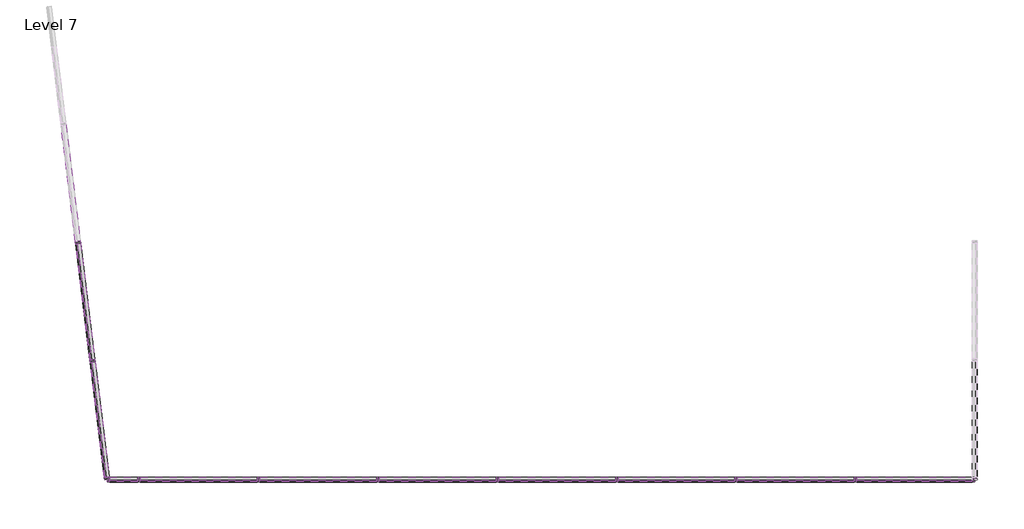
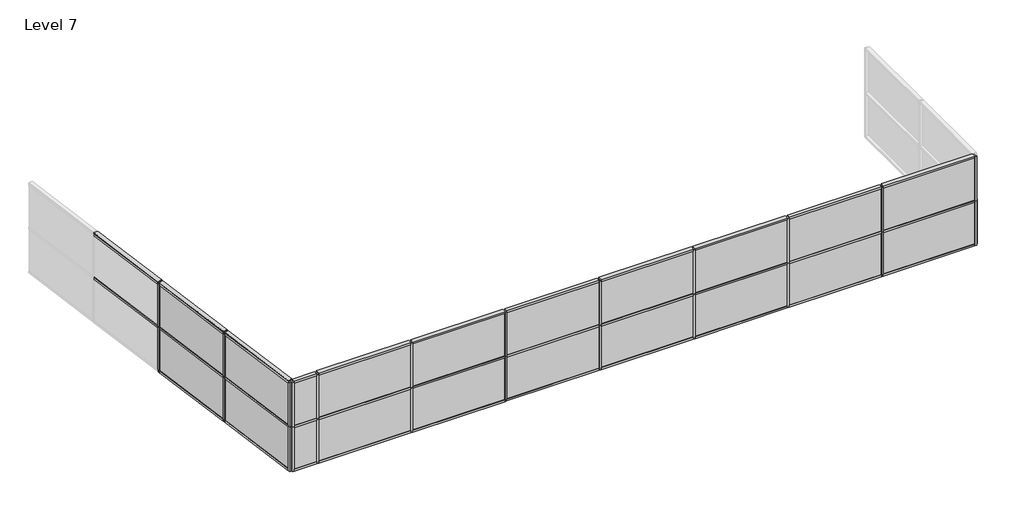
# One storey, part 1 of 2: 70 members, 24 plates.
"""IFC4 building model written with IfcOpenShell, lengths in millimetres."""

from ifc_helpers import new_model, si_unit, origin, place, context, project, spatial, transform, mapped, element, save
from components import member_71c27fd2, member_daa7a266, member_82905deb, member_19d0a4ec, member_8cef0660, member_db480205, member_4491d118, member_695b83e4, member_0c11e56c, system_panel_glazed_37f15d2e, system_panel_glazed_3620f98e, system_panel_glazed_e46d4b42, system_panel_glazed_2a6c68b7, system_panel_glazed_07b088f8, system_panel_glazed_9d0e0944

model = new_model("IFC4")

# Units and contexts
model_context = context("Model", 3, world=origin())
ifc_project = project(units=[si_unit("LENGTHUNIT", "METRE", prefix="MILLI")], contexts=[model_context])

# Site, building, storey
site = spatial("IfcSite", under=ifc_project)
building = spatial("IfcBuilding", under=site)
storey = spatial("IfcBuildingStorey", under=building, Name="Level 7", Elevation=18288.0)

# Members
placement = place(None, origin())
member_shape = member_71c27fd2(model_context)
element("IfcMember", 1, ObjectType="Rectangular Mullion : 2.5\" x 5\" rectangular", at=placement, inside=storey, context=model_context, shape_type="MappedRepresentation", body=[
    mapped(member_shape, transform((10886.265636, -6979.1363705, 18288.0), x_axis=(0.0, 0.0, -1.0), y_axis=(0.0, -1.0, 0.0), z_axis=(-1.0, 0.0, 0.0))),
])
element("IfcMember", 2, ObjectType="Rectangular Mullion : 2.5\" x 5\" rectangular", at=placement, inside=storey, context=model_context, shape_type="MappedRepresentation", body=[
    mapped(member_shape, transform((-8620.3262186, -3985.3690403, 18288.0), x_axis=(0.0, 0.0, -1.0), y_axis=(-0.9925461516413222, -0.12186934340514607, 0.0), z_axis=(-0.12186934340514607, 0.9925461516413222, 0.0))),
])
element("IfcMember", 3, ObjectType="Rectangular Mullion : 2.5\" x 5\" rectangular", at=placement, inside=storey, context=model_context, shape_type="MappedRepresentation", body=[
    mapped(member_shape, transform((13902.5156363, -6915.6363705, 18288.0), x_axis=(0.0, 0.0, -1.0), y_axis=(1.0, 0.0, 0.0), z_axis=(0.0, -1.0, 0.0))),
])
member_2_shape = member_daa7a266(model_context)
element("IfcMember", 4, ObjectType="Rectangular Mullion : 2.5\" x 5\" rectangular", at=placement, inside=storey, context=model_context, shape_type="MappedRepresentation", body=[
    mapped(member_2_shape, transform((-8260.4765148, -6916.1096898, 21336.0), x_axis=(0.0, 0.0, 1.0), y_axis=(-0.9925461516413222, -0.12186934340514587, 0.0), z_axis=(0.12186934340514587, -0.9925461516413222, 0.0))),
])
member_3_shape = member_82905deb(model_context)
element("IfcMember", 5, ObjectType="Rectangular Mullion : 2.5\" x 5\" rectangular", at=placement, inside=storey, context=model_context, shape_type="MappedRepresentation", body=[
    mapped(member_3_shape, transform((-8624.1955702, -3953.8557, 21336.0), x_axis=(-0.1218693434051459, 0.9925461516413222, 0.0), y_axis=(-0.9925461516413222, -0.1218693434051459, 0.0), z_axis=(0.0, 0.0, 1.0))),
])
element("IfcMember", 6, ObjectType="Rectangular Mullion : 2.5\" x 5\" rectangular", at=placement, inside=storey, context=model_context, shape_type="MappedRepresentation", body=[
    mapped(member_3_shape, transform((-8995.6533289, -928.5750297, 21336.0), x_axis=(-0.1218693434051459, 0.9925461516413222, 0.0), y_axis=(-0.9925461516413222, -0.1218693434051459, 0.0), z_axis=(0.0, 0.0, 1.0))),
])
member_4_shape = member_19d0a4ec(model_context)
element("IfcMember", 7, ObjectType="Rectangular Mullion : 2.5\" x 5\" rectangular", at=placement, inside=storey, context=model_context, shape_type="MappedRepresentation", body=[
    mapped(member_4_shape, transform((13839.0156363, -6979.1363705, 19812.0), x_axis=(0.0, 0.0, 1.0), y_axis=(0.0, -1.0, 0.0), z_axis=(1.0, 0.0, 0.0))),
])
element("IfcMember", 8, ObjectType="Rectangular Mullion : 2.5\" x 5\" rectangular", at=placement, inside=storey, context=model_context, shape_type="MappedRepresentation", body=[
    mapped(member_4_shape, transform((13839.0156363, -6979.1363705, 21336.0), x_axis=(0.0, 0.0, 1.0), y_axis=(0.0, -1.0, 0.0), z_axis=(1.0, 0.0, 0.0))),
])
element("IfcMember", 9, ObjectType="Rectangular Mullion : 2.5\" x 5\" rectangular", at=placement, inside=storey, context=model_context, shape_type="MappedRepresentation", body=[
    mapped(member_4_shape, transform((-8260.4765148, -6916.1096898, 19812.0), x_axis=(0.0, 0.0, 1.0), y_axis=(-0.9925461516413222, -0.12186934340514567, 0.0), z_axis=(0.12186934340514567, -0.9925461516413222, 0.0))),
])
element("IfcMember", 10, ObjectType="Rectangular Mullion : 2.5\" x 5\" rectangular", at=placement, inside=storey, context=model_context, shape_type="MappedRepresentation", body=[
    mapped(member_4_shape, transform((-8260.4765148, -6916.1096898, 19812.0), x_axis=(0.0, 0.0, 1.0), y_axis=(-0.9925461516413222, -0.12186934340514587, 0.0), z_axis=(0.12186934340514587, -0.9925461516413222, 0.0))),
])
element("IfcMember", 11, ObjectType="Rectangular Mullion : 2.5\" x 5\" rectangular", at=placement, inside=storey, context=model_context, shape_type="MappedRepresentation", body=[
    mapped(member_4_shape, transform((-8260.4765148, -6916.1096898, 21336.0), x_axis=(0.0, 0.0, 1.0), y_axis=(-0.9925461516413223, -0.12186934340514574, 0.0), z_axis=(0.12186934340514574, -0.9925461516413223, 0.0))),
])
member_5_shape = member_8cef0660(model_context)
element("IfcMember", 12, ObjectType="Rectangular Mullion : 2.5\" x 5\" rectangular", at=placement, inside=storey, context=model_context, shape_type="MappedRepresentation", body=[
    mapped(member_5_shape, transform((10822.765636, -6979.1363705, 19812.0), x_axis=(0.0, 0.0, 1.0), y_axis=(0.0, -1.0, 0.0), z_axis=(1.0, 0.0, 0.0))),
])
element("IfcMember", 13, ObjectType="Rectangular Mullion : 2.5\" x 5\" rectangular", at=placement, inside=storey, context=model_context, shape_type="MappedRepresentation", body=[
    mapped(member_5_shape, transform((7774.765636, -6979.1363705, 19812.0), x_axis=(0.0, 0.0, 1.0), y_axis=(0.0, -1.0, 0.0), z_axis=(1.0, 0.0, 0.0))),
])
element("IfcMember", 14, ObjectType="Rectangular Mullion : 2.5\" x 5\" rectangular", at=placement, inside=storey, context=model_context, shape_type="MappedRepresentation", body=[
    mapped(member_5_shape, transform((4726.765636, -6979.1363705, 19812.0), x_axis=(0.0, 0.0, 1.0), y_axis=(0.0, -1.0, 0.0), z_axis=(1.0, 0.0, 0.0))),
])
element("IfcMember", 15, ObjectType="Rectangular Mullion : 2.5\" x 5\" rectangular", at=placement, inside=storey, context=model_context, shape_type="MappedRepresentation", body=[
    mapped(member_5_shape, transform((1678.765636, -6979.1363705, 19812.0), x_axis=(0.0, 0.0, 1.0), y_axis=(0.0, -1.0, 0.0), z_axis=(1.0, 0.0, 0.0))),
])
element("IfcMember", 16, ObjectType="Rectangular Mullion : 2.5\" x 5\" rectangular", at=placement, inside=storey, context=model_context, shape_type="MappedRepresentation", body=[
    mapped(member_5_shape, transform((-1369.234364, -6979.1363705, 19812.0), x_axis=(0.0, 0.0, 1.0), y_axis=(0.0, -1.0, 0.0), z_axis=(1.0, 0.0, 0.0))),
])
element("IfcMember", 17, ObjectType="Rectangular Mullion : 2.5\" x 5\" rectangular", at=placement, inside=storey, context=model_context, shape_type="MappedRepresentation", body=[
    mapped(member_5_shape, transform((-4417.234364, -6979.1363705, 19812.0), x_axis=(0.0, 0.0, 1.0), y_axis=(0.0, -1.0, 0.0), z_axis=(1.0, 0.0, 0.0))),
])
element("IfcMember", 18, ObjectType="Rectangular Mullion : 2.5\" x 5\" rectangular", at=placement, inside=storey, context=model_context, shape_type="MappedRepresentation", body=[
    mapped(member_5_shape, transform((10822.765636, -6979.1363705, 21336.0), x_axis=(0.0, 0.0, 1.0), y_axis=(0.0, -1.0, 0.0), z_axis=(1.0, 0.0, 0.0))),
])
element("IfcMember", 19, ObjectType="Rectangular Mullion : 2.5\" x 5\" rectangular", at=placement, inside=storey, context=model_context, shape_type="MappedRepresentation", body=[
    mapped(member_5_shape, transform((7774.765636, -6979.1363705, 21336.0), x_axis=(0.0, 0.0, 1.0), y_axis=(0.0, -1.0, 0.0), z_axis=(1.0, 0.0, 0.0))),
])
element("IfcMember", 20, ObjectType="Rectangular Mullion : 2.5\" x 5\" rectangular", at=placement, inside=storey, context=model_context, shape_type="MappedRepresentation", body=[
    mapped(member_5_shape, transform((4726.765636, -6979.1363705, 21336.0), x_axis=(0.0, 0.0, 1.0), y_axis=(0.0, -1.0, 0.0), z_axis=(1.0, 0.0, 0.0))),
])
element("IfcMember", 21, ObjectType="Rectangular Mullion : 2.5\" x 5\" rectangular", at=placement, inside=storey, context=model_context, shape_type="MappedRepresentation", body=[
    mapped(member_5_shape, transform((1678.765636, -6979.1363705, 21336.0), x_axis=(0.0, 0.0, 1.0), y_axis=(0.0, -1.0, 0.0), z_axis=(1.0, 0.0, 0.0))),
])
element("IfcMember", 22, ObjectType="Rectangular Mullion : 2.5\" x 5\" rectangular", at=placement, inside=storey, context=model_context, shape_type="MappedRepresentation", body=[
    mapped(member_5_shape, transform((-1369.234364, -6979.1363705, 21336.0), x_axis=(0.0, 0.0, 1.0), y_axis=(0.0, -1.0, 0.0), z_axis=(1.0, 0.0, 0.0))),
])
element("IfcMember", 23, ObjectType="Rectangular Mullion : 2.5\" x 5\" rectangular", at=placement, inside=storey, context=model_context, shape_type="MappedRepresentation", body=[
    mapped(member_5_shape, transform((-4417.234364, -6979.1363705, 21336.0), x_axis=(0.0, 0.0, 1.0), y_axis=(0.0, -1.0, 0.0), z_axis=(1.0, 0.0, 0.0))),
])
element("IfcMember", 24, ObjectType="Rectangular Mullion : 2.5\" x 5\" rectangular", at=placement, inside=storey, context=model_context, shape_type="MappedRepresentation", body=[
    mapped(member_5_shape, transform((-8628.0649219, -3922.3423596, 19812.0), x_axis=(0.0, 0.0, 1.0), y_axis=(-0.9925461516413222, -0.12186934340514595, 0.0), z_axis=(0.12186934340514595, -0.9925461516413222, 0.0))),
])
element("IfcMember", 25, ObjectType="Rectangular Mullion : 2.5\" x 5\" rectangular", at=placement, inside=storey, context=model_context, shape_type="MappedRepresentation", body=[
    mapped(member_5_shape, transform((-8999.5226806, -897.0616894, 19812.0), x_axis=(0.0, 0.0, 1.0), y_axis=(-0.9925461516413222, -0.12186934340514599, 0.0), z_axis=(0.12186934340514599, -0.9925461516413222, 0.0))),
])
element("IfcMember", 26, ObjectType="Rectangular Mullion : 2.5\" x 5\" rectangular", at=placement, inside=storey, context=model_context, shape_type="MappedRepresentation", body=[
    mapped(member_5_shape, transform((-8628.0649219, -3922.3423596, 19812.0), x_axis=(0.0, 0.0, 1.0), y_axis=(-0.9925461516413222, -0.1218693434051457, 0.0), z_axis=(0.1218693434051457, -0.9925461516413222, 0.0))),
])
element("IfcMember", 27, ObjectType="Rectangular Mullion : 2.5\" x 5\" rectangular", at=placement, inside=storey, context=model_context, shape_type="MappedRepresentation", body=[
    mapped(member_5_shape, transform((-8999.5226806, -897.0616894, 19812.0), x_axis=(0.0, 0.0, 1.0), y_axis=(-0.9925461516413222, -0.12186934340514596, 0.0), z_axis=(0.12186934340514596, -0.9925461516413222, 0.0))),
])
element("IfcMember", 28, ObjectType="Rectangular Mullion : 2.5\" x 5\" rectangular", at=placement, inside=storey, context=model_context, shape_type="MappedRepresentation", body=[
    mapped(member_5_shape, transform((-8628.0649219, -3922.3423596, 21336.0), x_axis=(0.0, 0.0, 1.0), y_axis=(-0.9925461516413222, -0.12186934340514606, 0.0), z_axis=(0.12186934340514606, -0.9925461516413222, 0.0))),
])
element("IfcMember", 29, ObjectType="Rectangular Mullion : 2.5\" x 5\" rectangular", at=placement, inside=storey, context=model_context, shape_type="MappedRepresentation", body=[
    mapped(member_5_shape, transform((-8999.5226806, -897.0616894, 21336.0), x_axis=(0.0, 0.0, 1.0), y_axis=(-0.9925461516413222, -0.12186934340514595, 0.0), z_axis=(0.12186934340514595, -0.9925461516413222, 0.0))),
])
member_6_shape = member_db480205(model_context)
element("IfcMember", 30, ObjectType="Rectangular Mullion : 2.5\" x 5\" rectangular", at=placement, inside=storey, context=model_context, shape_type="MappedRepresentation", body=[
    mapped(member_6_shape, transform((7838.265636, -6979.1363705, 18288.0), x_axis=(0.0, 0.0, -1.0), y_axis=(0.0, -1.0, 0.0), z_axis=(-1.0, 0.0, 0.0))),
])
element("IfcMember", 31, ObjectType="Rectangular Mullion : 2.5\" x 5\" rectangular", at=placement, inside=storey, context=model_context, shape_type="MappedRepresentation", body=[
    mapped(member_6_shape, transform((4790.265636, -6979.1363705, 18288.0), x_axis=(0.0, 0.0, -1.0), y_axis=(0.0, -1.0, 0.0), z_axis=(-1.0, 0.0, 0.0))),
])
element("IfcMember", 32, ObjectType="Rectangular Mullion : 2.5\" x 5\" rectangular", at=placement, inside=storey, context=model_context, shape_type="MappedRepresentation", body=[
    mapped(member_6_shape, transform((1742.265636, -6979.1363705, 18288.0), x_axis=(0.0, 0.0, -1.0), y_axis=(0.0, -1.0, 0.0), z_axis=(-1.0, 0.0, 0.0))),
])
element("IfcMember", 33, ObjectType="Rectangular Mullion : 2.5\" x 5\" rectangular", at=placement, inside=storey, context=model_context, shape_type="MappedRepresentation", body=[
    mapped(member_6_shape, transform((-1305.734364, -6979.1363705, 18288.0), x_axis=(0.0, 0.0, -1.0), y_axis=(0.0, -1.0, 0.0), z_axis=(-1.0, 0.0, 0.0))),
])
element("IfcMember", 34, ObjectType="Rectangular Mullion : 2.5\" x 5\" rectangular", at=placement, inside=storey, context=model_context, shape_type="MappedRepresentation", body=[
    mapped(member_6_shape, transform((-4353.734364, -6979.1363705, 18288.0), x_axis=(0.0, 0.0, -1.0), y_axis=(0.0, -1.0, 0.0), z_axis=(-1.0, 0.0, 0.0))),
])
element("IfcMember", 35, ObjectType="Rectangular Mullion : 2.5\" x 5\" rectangular", at=placement, inside=storey, context=model_context, shape_type="MappedRepresentation", body=[
    mapped(member_6_shape, transform((-7401.734364, -6979.1363705, 18288.0), x_axis=(0.0, 0.0, -1.0), y_axis=(0.0, -1.0, 0.0), z_axis=(-1.0, 0.0, 0.0))),
])
element("IfcMember", 36, ObjectType="Rectangular Mullion : 2.5\" x 5\" rectangular", at=placement, inside=storey, context=model_context, shape_type="MappedRepresentation", body=[
    mapped(member_6_shape, transform((-8991.7839773, -960.0883701, 18288.0), x_axis=(0.0, 0.0, -1.0), y_axis=(-0.9925461516413222, -0.12186934340514607, 0.0), z_axis=(-0.12186934340514607, 0.9925461516413222, 0.0))),
])
element("IfcMember", 37, ObjectType="Rectangular Mullion : 2.5\" x 5\" rectangular", at=placement, inside=storey, context=model_context, shape_type="MappedRepresentation", body=[
    mapped(member_6_shape, transform((-8628.0649219, -3922.3423596, 21336.0), x_axis=(0.0, 0.0, 1.0), y_axis=(-0.9925461516413222, -0.12186934340514592, 0.0), z_axis=(0.12186934340514592, -0.9925461516413222, 0.0))),
])
element("IfcMember", 38, ObjectType="Rectangular Mullion : 2.5\" x 5\" rectangular", at=placement, inside=storey, context=model_context, shape_type="MappedRepresentation", body=[
    mapped(member_6_shape, transform((-8999.5226806, -897.0616894, 21336.0), x_axis=(0.0, 0.0, 1.0), y_axis=(-0.9925461516413222, -0.12186934340514596, 0.0), z_axis=(0.12186934340514596, -0.9925461516413222, 0.0))),
])
element("IfcMember", 39, ObjectType="Rectangular Mullion : 2.5\" x 5\" rectangular", at=placement, inside=storey, context=model_context, shape_type="MappedRepresentation", body=[
    mapped(member_3_shape, transform((10854.515636, -6979.1363705, 19812.0), x_axis=(-1.0, 0.0, 0.0), y_axis=(0.0, -1.0, 0.0), z_axis=(0.0, 0.0, 1.0))),
])
element("IfcMember", 40, ObjectType="Rectangular Mullion : 2.5\" x 5\" rectangular", at=placement, inside=storey, context=model_context, shape_type="MappedRepresentation", body=[
    mapped(member_3_shape, transform((7806.515636, -6979.1363705, 19812.0), x_axis=(-1.0, 0.0, 0.0), y_axis=(0.0, -1.0, 0.0), z_axis=(0.0, 0.0, 1.0))),
])
element("IfcMember", 41, ObjectType="Rectangular Mullion : 2.5\" x 5\" rectangular", at=placement, inside=storey, context=model_context, shape_type="MappedRepresentation", body=[
    mapped(member_3_shape, transform((4758.515636, -6979.1363705, 19812.0), x_axis=(-1.0, 0.0, 0.0), y_axis=(0.0, -1.0, 0.0), z_axis=(0.0, 0.0, 1.0))),
])
element("IfcMember", 42, ObjectType="Rectangular Mullion : 2.5\" x 5\" rectangular", at=placement, inside=storey, context=model_context, shape_type="MappedRepresentation", body=[
    mapped(member_3_shape, transform((1710.515636, -6979.1363705, 19812.0), x_axis=(-1.0, 0.0, 0.0), y_axis=(0.0, -1.0, 0.0), z_axis=(0.0, 0.0, 1.0))),
])
element("IfcMember", 43, ObjectType="Rectangular Mullion : 2.5\" x 5\" rectangular", at=placement, inside=storey, context=model_context, shape_type="MappedRepresentation", body=[
    mapped(member_3_shape, transform((-1337.484364, -6979.1363705, 19812.0), x_axis=(-1.0, 0.0, 0.0), y_axis=(0.0, -1.0, 0.0), z_axis=(0.0, 0.0, 1.0))),
])
element("IfcMember", 44, ObjectType="Rectangular Mullion : 2.5\" x 5\" rectangular", at=placement, inside=storey, context=model_context, shape_type="MappedRepresentation", body=[
    mapped(member_3_shape, transform((-4385.484364, -6979.1363705, 19812.0), x_axis=(-1.0, 0.0, 0.0), y_axis=(0.0, -1.0, 0.0), z_axis=(0.0, 0.0, 1.0))),
])
element("IfcMember", 45, ObjectType="Rectangular Mullion : 2.5\" x 5\" rectangular", at=placement, inside=storey, context=model_context, shape_type="MappedRepresentation", body=[
    mapped(member_3_shape, transform((-7433.484364, -6979.1363705, 19812.0), x_axis=(-1.0, 0.0, 0.0), y_axis=(0.0, -1.0, 0.0), z_axis=(0.0, 0.0, 1.0))),
])
element("IfcMember", 46, ObjectType="Rectangular Mullion : 2.5\" x 5\" rectangular", at=placement, inside=storey, context=model_context, shape_type="MappedRepresentation", body=[
    mapped(member_3_shape, transform((-8624.1955702, -3953.8557, 19812.0), x_axis=(-0.1218693434051459, 0.9925461516413222, 0.0), y_axis=(-0.9925461516413222, -0.1218693434051459, 0.0), z_axis=(0.0, 0.0, 1.0))),
])
element("IfcMember", 47, ObjectType="Rectangular Mullion : 2.5\" x 5\" rectangular", at=placement, inside=storey, context=model_context, shape_type="MappedRepresentation", body=[
    mapped(member_3_shape, transform((-8995.6533289, -928.5750297, 19812.0), x_axis=(-0.1218693434051459, 0.9925461516413222, 0.0), y_axis=(-0.9925461516413222, -0.1218693434051459, 0.0), z_axis=(0.0, 0.0, 1.0))),
])
element("IfcMember", 48, ObjectType="Rectangular Mullion : 2.5\" x 5\" rectangular", at=placement, inside=storey, context=model_context, shape_type="MappedRepresentation", body=[
    mapped(member_3_shape, transform((10854.515636, -6979.1363705, 21336.0), x_axis=(-1.0, 0.0, 0.0), y_axis=(0.0, -1.0, 0.0), z_axis=(0.0, 0.0, 1.0))),
])
element("IfcMember", 49, ObjectType="Rectangular Mullion : 2.5\" x 5\" rectangular", at=placement, inside=storey, context=model_context, shape_type="MappedRepresentation", body=[
    mapped(member_3_shape, transform((7806.515636, -6979.1363705, 21336.0), x_axis=(-1.0, 0.0, 0.0), y_axis=(0.0, -1.0, 0.0), z_axis=(0.0, 0.0, 1.0))),
])
element("IfcMember", 50, ObjectType="Rectangular Mullion : 2.5\" x 5\" rectangular", at=placement, inside=storey, context=model_context, shape_type="MappedRepresentation", body=[
    mapped(member_3_shape, transform((4758.515636, -6979.1363705, 21336.0), x_axis=(-1.0, 0.0, 0.0), y_axis=(0.0, -1.0, 0.0), z_axis=(0.0, 0.0, 1.0))),
])
element("IfcMember", 51, ObjectType="Rectangular Mullion : 2.5\" x 5\" rectangular", at=placement, inside=storey, context=model_context, shape_type="MappedRepresentation", body=[
    mapped(member_3_shape, transform((1710.515636, -6979.1363705, 21336.0), x_axis=(-1.0, 0.0, 0.0), y_axis=(0.0, -1.0, 0.0), z_axis=(0.0, 0.0, 1.0))),
])
element("IfcMember", 52, ObjectType="Rectangular Mullion : 2.5\" x 5\" rectangular", at=placement, inside=storey, context=model_context, shape_type="MappedRepresentation", body=[
    mapped(member_3_shape, transform((-1337.484364, -6979.1363705, 21336.0), x_axis=(-1.0, 0.0, 0.0), y_axis=(0.0, -1.0, 0.0), z_axis=(0.0, 0.0, 1.0))),
])
element("IfcMember", 53, ObjectType="Rectangular Mullion : 2.5\" x 5\" rectangular", at=placement, inside=storey, context=model_context, shape_type="MappedRepresentation", body=[
    mapped(member_3_shape, transform((-4385.484364, -6979.1363705, 21336.0), x_axis=(-1.0, 0.0, 0.0), y_axis=(0.0, -1.0, 0.0), z_axis=(0.0, 0.0, 1.0))),
])
element("IfcMember", 54, ObjectType="Rectangular Mullion : 2.5\" x 5\" rectangular", at=placement, inside=storey, context=model_context, shape_type="MappedRepresentation", body=[
    mapped(member_3_shape, transform((-7433.484364, -6979.1363705, 21336.0), x_axis=(-1.0, 0.0, 0.0), y_axis=(0.0, -1.0, 0.0), z_axis=(0.0, 0.0, 1.0))),
])
element("IfcMember", 55, ObjectType="Rectangular Mullion : 2.5\" x 5\" rectangular", at=placement, inside=storey, context=model_context, shape_type="MappedRepresentation", body=[
    mapped(member_3_shape, transform((-8624.1955702, -3953.8557, 19812.0), x_axis=(-0.1218693434051459, 0.9925461516413222, 0.0), y_axis=(-0.9925461516413222, -0.1218693434051459, 0.0), z_axis=(0.0, 0.0, 1.0))),
])
element("IfcMember", 56, ObjectType="Rectangular Mullion : 2.5\" x 5\" rectangular", at=placement, inside=storey, context=model_context, shape_type="MappedRepresentation", body=[
    mapped(member_3_shape, transform((-8995.6533289, -928.5750297, 19812.0), x_axis=(-0.1218693434051459, 0.9925461516413222, 0.0), y_axis=(-0.9925461516413222, -0.1218693434051459, 0.0), z_axis=(0.0, 0.0, 1.0))),
])
element("IfcMember", 57, ObjectType="Rectangular Mullion : 2.5\" x 5\" rectangular", at=placement, inside=storey, context=model_context, shape_type="MappedRepresentation", body=[
    mapped(member_3_shape, transform((-8624.1955702, -3953.8557, 21336.0), x_axis=(-0.1218693434051459, 0.9925461516413222, 0.0), y_axis=(-0.9925461516413222, -0.1218693434051459, 0.0), z_axis=(0.0, 0.0, 1.0))),
])
element("IfcMember", 58, ObjectType="Rectangular Mullion : 2.5\" x 5\" rectangular", at=placement, inside=storey, context=model_context, shape_type="MappedRepresentation", body=[
    mapped(member_3_shape, transform((-8995.6533289, -928.5750297, 21336.0), x_axis=(-0.1218693434051459, 0.9925461516413222, 0.0), y_axis=(-0.9925461516413222, -0.1218693434051459, 0.0), z_axis=(0.0, 0.0, 1.0))),
])
member_7_shape = member_4491d118(model_context)
element("IfcMember", 59, ObjectType="Rectangular Mullion : 2.5\" x 5\" rectangular", at=placement, inside=storey, context=model_context, shape_type="MappedRepresentation", body=[
    mapped(member_7_shape, transform((13902.5156363, -6979.1363705, 18288.0), x_axis=(1.0, 0.0, 0.0), y_axis=(0.0, -1.0, 0.0), z_axis=(0.0, 0.0, -1.0))),
])
element("IfcMember", 60, ObjectType="Rectangular Mullion : 2.5\" x 5\" rectangular", at=placement, inside=storey, context=model_context, shape_type="MappedRepresentation", body=[
    mapped(member_7_shape, transform((-8252.7378115, -6979.1363705, 18288.0), x_axis=(0.1218693434051459, -0.9925461516413222, 0.0), y_axis=(-0.9925461516413222, -0.1218693434051459, 0.0), z_axis=(0.0, 0.0, -1.0))),
])
element("IfcMember", 61, ObjectType="Rectangular Mullion : 2.5\" x 5\" rectangular", at=placement, inside=storey, context=model_context, shape_type="MappedRepresentation", body=[
    mapped(member_7_shape, transform((13902.5156363, -6979.1363705, 19812.0), x_axis=(1.0, 0.0, 0.0), y_axis=(0.0, -1.0, 0.0), z_axis=(0.0, 0.0, -1.0))),
])
element("IfcMember", 62, ObjectType="Rectangular Mullion : 2.5\" x 5\" rectangular", at=placement, inside=storey, context=model_context, shape_type="MappedRepresentation", body=[
    mapped(member_7_shape, transform((-8252.7378115, -6979.1363705, 18288.0), x_axis=(0.1218693434051459, -0.9925461516413222, 0.0), y_axis=(-0.9925461516413222, -0.1218693434051459, 0.0), z_axis=(0.0, 0.0, -1.0))),
])
element("IfcMember", 63, ObjectType="Rectangular Mullion : 2.5\" x 5\" rectangular", at=placement, inside=storey, context=model_context, shape_type="MappedRepresentation", body=[
    mapped(member_7_shape, transform((-8252.7378115, -6979.1363705, 19812.0), x_axis=(0.1218693434051459, -0.9925461516413222, 0.0), y_axis=(-0.9925461516413222, -0.1218693434051459, 0.0), z_axis=(0.0, 0.0, -1.0))),
])
element("IfcMember", 64, ObjectType="Rectangular Mullion : 2.5\" x 5\" rectangular", at=placement, inside=storey, context=model_context, shape_type="MappedRepresentation", body=[
    mapped(member_7_shape, transform((-8252.7378115, -6979.1363705, 19812.0), x_axis=(0.1218693434051459, -0.9925461516413222, 0.0), y_axis=(-0.9925461516413222, -0.1218693434051459, 0.0), z_axis=(0.0, 0.0, -1.0))),
])
element("IfcMember", 65, ObjectType="Rectangular Mullion : 2.5\" x 5\" rectangular", at=placement, inside=storey, context=model_context, shape_type="MappedRepresentation", body=[
    mapped(member_7_shape, transform((-8252.7378115, -6979.1363705, 19812.0), x_axis=(-1.0, 0.0, 0.0), y_axis=(0.0, -1.0, 0.0), z_axis=(0.0, 0.0, 1.0))),
])
element("IfcMember", 66, ObjectType="Rectangular Mullion : 2.5\" x 5\" rectangular", at=placement, inside=storey, context=model_context, shape_type="MappedRepresentation", body=[
    mapped(member_7_shape, transform((13902.5156363, -6979.1363705, 19812.0), x_axis=(0.0, -1.0, 0.0), y_axis=(1.0, 0.0, 0.0), z_axis=(0.0, 0.0, 1.0))),
])
element("IfcMember", 67, ObjectType="Rectangular Mullion : 2.5\" x 5\" rectangular", at=placement, inside=storey, context=model_context, shape_type="MappedRepresentation", body=[
    mapped(member_7_shape, transform((-8252.7378115, -6979.1363705, 21336.0), x_axis=(-1.0, 0.0, 0.0), y_axis=(0.0, -1.0, 0.0), z_axis=(0.0, 0.0, 1.0))),
])
member_8_shape = member_695b83e4(model_context)
element("IfcMember", 68, ObjectType="Rectangular Mullion : 2.5\" x 5\" rectangular", at=placement, inside=storey, context=model_context, shape_type="MappedRepresentation", body=[
    mapped(member_8_shape, transform((-8189.2378115, -6979.1363705, 18288.0), x_axis=(0.0, 0.0, -1.0), y_axis=(0.0, -1.0, 0.0), z_axis=(-1.0, 0.0, 0.0))),
])
member_9_shape = member_0c11e56c(model_context)
element("IfcMember", 69, ObjectType="Rectangular Mullion : 2.5\" x 5\" rectangular", at=placement, inside=storey, context=model_context, shape_type="MappedRepresentation", body=[
    mapped(member_9_shape, transform((-7465.234364, -6979.1363705, 19812.0), x_axis=(0.0, 0.0, 1.0), y_axis=(0.0, -1.0, 0.0), z_axis=(1.0, 0.0, 0.0))),
])
element("IfcMember", 70, ObjectType="Rectangular Mullion : 2.5\" x 5\" rectangular", at=placement, inside=storey, context=model_context, shape_type="MappedRepresentation", body=[
    mapped(member_9_shape, transform((-7465.234364, -6979.1363705, 21336.0), x_axis=(0.0, 0.0, 1.0), y_axis=(0.0, -1.0, 0.0), z_axis=(1.0, 0.0, 0.0))),
])

# Plates
system_panel_glazed_shape = system_panel_glazed_37f15d2e(model_context)
element("IfcPlate", 71, ObjectType="System Panel : Glazed", at=placement, inside=storey, context=model_context, shape_type="MappedRepresentation", body=[
    mapped(system_panel_glazed_shape, transform((-8440.4013667, -5450.739365, 18351.5), x_axis=(-0.1218693434051459, 0.9925461516413222, 0.0), y_axis=(-0.9925461516413222, -0.1218693434051459, 0.0), z_axis=(0.0, 0.0, 1.0))),
])
element("IfcPlate", 72, ObjectType="System Panel : Glazed", at=placement, inside=storey, context=model_context, shape_type="MappedRepresentation", body=[
    mapped(system_panel_glazed_shape, transform((12362.6406361, -6979.1363705, 18351.5), x_axis=(-1.0, 0.0, 0.0), y_axis=(0.0, -1.0, 0.0), z_axis=(0.0, 0.0, 1.0))),
])
element("IfcPlate", 73, ObjectType="System Panel : Glazed", at=placement, inside=storey, context=model_context, shape_type="MappedRepresentation", body=[
    mapped(system_panel_glazed_shape, transform((-8440.4013667, -5450.739365, 19843.75), x_axis=(-0.1218693434051459, 0.9925461516413222, 0.0), y_axis=(-0.9925461516413222, -0.1218693434051459, 0.0), z_axis=(0.0, 0.0, 1.0))),
])
system_panel_glazed_2_shape = system_panel_glazed_3620f98e(model_context)
element("IfcPlate", 74, ObjectType="System Panel : Glazed", at=placement, inside=storey, context=model_context, shape_type="MappedRepresentation", body=[
    mapped(system_panel_glazed_2_shape, transform((-8809.9244496, -2441.2153649, 19843.75), x_axis=(-0.1218693434051459, 0.9925461516413222, 0.0), y_axis=(-0.9925461516413222, -0.1218693434051459, 0.0), z_axis=(0.0, 0.0, 1.0))),
])
element("IfcPlate", 75, ObjectType="System Panel : Glazed", at=placement, inside=storey, context=model_context, shape_type="MappedRepresentation", body=[
    mapped(system_panel_glazed_2_shape, transform((-8809.9244496, -2441.2153649, 18351.5), x_axis=(-0.1218693434051459, 0.9925461516413222, 0.0), y_axis=(-0.9925461516413222, -0.1218693434051459, 0.0), z_axis=(0.0, 0.0, 1.0))),
])
element("IfcPlate", 76, ObjectType="System Panel : Glazed", at=placement, inside=storey, context=model_context, shape_type="MappedRepresentation", body=[
    mapped(system_panel_glazed_2_shape, transform((9330.515636, -6979.1363705, 18351.5), x_axis=(-1.0, 0.0, 0.0), y_axis=(0.0, -1.0, 0.0), z_axis=(0.0, 0.0, 1.0))),
])
element("IfcPlate", 77, ObjectType="System Panel : Glazed", at=placement, inside=storey, context=model_context, shape_type="MappedRepresentation", body=[
    mapped(system_panel_glazed_2_shape, transform((6282.515636, -6979.1363705, 18351.5), x_axis=(-1.0, 0.0, 0.0), y_axis=(0.0, -1.0, 0.0), z_axis=(0.0, 0.0, 1.0))),
])
element("IfcPlate", 78, ObjectType="System Panel : Glazed", at=placement, inside=storey, context=model_context, shape_type="MappedRepresentation", body=[
    mapped(system_panel_glazed_2_shape, transform((3234.515636, -6979.1363705, 18351.5), x_axis=(-1.0, 0.0, 0.0), y_axis=(0.0, -1.0, 0.0), z_axis=(0.0, 0.0, 1.0))),
])
element("IfcPlate", 79, ObjectType="System Panel : Glazed", at=placement, inside=storey, context=model_context, shape_type="MappedRepresentation", body=[
    mapped(system_panel_glazed_2_shape, transform((186.515636, -6979.1363705, 18351.5), x_axis=(-1.0, 0.0, 0.0), y_axis=(0.0, -1.0, 0.0), z_axis=(0.0, 0.0, 1.0))),
])
element("IfcPlate", 80, ObjectType="System Panel : Glazed", at=placement, inside=storey, context=model_context, shape_type="MappedRepresentation", body=[
    mapped(system_panel_glazed_2_shape, transform((-2861.484364, -6979.1363705, 18351.5), x_axis=(-1.0, 0.0, 0.0), y_axis=(0.0, -1.0, 0.0), z_axis=(0.0, 0.0, 1.0))),
])
element("IfcPlate", 81, ObjectType="System Panel : Glazed", at=placement, inside=storey, context=model_context, shape_type="MappedRepresentation", body=[
    mapped(system_panel_glazed_2_shape, transform((-5909.484364, -6979.1363705, 18351.5), x_axis=(-1.0, 0.0, 0.0), y_axis=(0.0, -1.0, 0.0), z_axis=(0.0, 0.0, 1.0))),
])
system_panel_glazed_3_shape = system_panel_glazed_e46d4b42(model_context)
element("IfcPlate", 82, ObjectType="System Panel : Glazed", at=placement, inside=storey, context=model_context, shape_type="MappedRepresentation", body=[
    mapped(system_panel_glazed_3_shape, transform((-8440.4013667, -5450.739365, 18319.75), x_axis=(-0.1218693434051459, 0.9925461516413222, 0.0), y_axis=(-0.9925461516413222, -0.1218693434051459, 0.0), z_axis=(0.0, 0.0, 1.0))),
])
element("IfcPlate", 83, ObjectType="System Panel : Glazed", at=placement, inside=storey, context=model_context, shape_type="MappedRepresentation", body=[
    mapped(system_panel_glazed_3_shape, transform((-8440.4013667, -5450.739365, 19843.75), x_axis=(-0.1218693434051459, 0.9925461516413222, 0.0), y_axis=(-0.9925461516413222, -0.1218693434051459, 0.0), z_axis=(0.0, 0.0, 1.0))),
])
element("IfcPlate", 84, ObjectType="System Panel : Glazed", at=placement, inside=storey, context=model_context, shape_type="MappedRepresentation", body=[
    mapped(system_panel_glazed_3_shape, transform((12362.6406361, -6979.1363705, 19843.75), x_axis=(-1.0, 0.0, 0.0), y_axis=(0.0, -1.0, 0.0), z_axis=(0.0, 0.0, 1.0))),
])
system_panel_glazed_4_shape = system_panel_glazed_2a6c68b7(model_context)
element("IfcPlate", 85, ObjectType="System Panel : Glazed", at=placement, inside=storey, context=model_context, shape_type="MappedRepresentation", body=[
    mapped(system_panel_glazed_4_shape, transform((-8809.9244496, -2441.2153649, 18319.75), x_axis=(-0.1218693434051459, 0.9925461516413222, 0.0), y_axis=(-0.9925461516413222, -0.1218693434051459, 0.0), z_axis=(0.0, 0.0, 1.0))),
])
element("IfcPlate", 86, ObjectType="System Panel : Glazed", at=placement, inside=storey, context=model_context, shape_type="MappedRepresentation", body=[
    mapped(system_panel_glazed_4_shape, transform((-8809.9244496, -2441.2153649, 19843.75), x_axis=(-0.1218693434051459, 0.9925461516413222, 0.0), y_axis=(-0.9925461516413222, -0.1218693434051459, 0.0), z_axis=(0.0, 0.0, 1.0))),
])
element("IfcPlate", 87, ObjectType="System Panel : Glazed", at=placement, inside=storey, context=model_context, shape_type="MappedRepresentation", body=[
    mapped(system_panel_glazed_4_shape, transform((9330.515636, -6979.1363705, 19843.75), x_axis=(-1.0, 0.0, 0.0), y_axis=(0.0, -1.0, 0.0), z_axis=(0.0, 0.0, 1.0))),
])
element("IfcPlate", 88, ObjectType="System Panel : Glazed", at=placement, inside=storey, context=model_context, shape_type="MappedRepresentation", body=[
    mapped(system_panel_glazed_4_shape, transform((6282.515636, -6979.1363705, 19843.75), x_axis=(-1.0, 0.0, 0.0), y_axis=(0.0, -1.0, 0.0), z_axis=(0.0, 0.0, 1.0))),
])
element("IfcPlate", 89, ObjectType="System Panel : Glazed", at=placement, inside=storey, context=model_context, shape_type="MappedRepresentation", body=[
    mapped(system_panel_glazed_4_shape, transform((3234.515636, -6979.1363705, 19843.75), x_axis=(-1.0, 0.0, 0.0), y_axis=(0.0, -1.0, 0.0), z_axis=(0.0, 0.0, 1.0))),
])
element("IfcPlate", 90, ObjectType="System Panel : Glazed", at=placement, inside=storey, context=model_context, shape_type="MappedRepresentation", body=[
    mapped(system_panel_glazed_4_shape, transform((186.515636, -6979.1363705, 19843.75), x_axis=(-1.0, 0.0, 0.0), y_axis=(0.0, -1.0, 0.0), z_axis=(0.0, 0.0, 1.0))),
])
element("IfcPlate", 91, ObjectType="System Panel : Glazed", at=placement, inside=storey, context=model_context, shape_type="MappedRepresentation", body=[
    mapped(system_panel_glazed_4_shape, transform((-2861.484364, -6979.1363705, 19843.75), x_axis=(-1.0, 0.0, 0.0), y_axis=(0.0, -1.0, 0.0), z_axis=(0.0, 0.0, 1.0))),
])
element("IfcPlate", 92, ObjectType="System Panel : Glazed", at=placement, inside=storey, context=model_context, shape_type="MappedRepresentation", body=[
    mapped(system_panel_glazed_4_shape, transform((-5909.484364, -6979.1363705, 19843.75), x_axis=(-1.0, 0.0, 0.0), y_axis=(0.0, -1.0, 0.0), z_axis=(0.0, 0.0, 1.0))),
])
system_panel_glazed_5_shape = system_panel_glazed_07b088f8(model_context)
element("IfcPlate", 93, ObjectType="System Panel : Glazed", at=placement, inside=storey, context=model_context, shape_type="MappedRepresentation", body=[
    mapped(system_panel_glazed_5_shape, transform((-7827.2360878, -6979.1363705, 18351.5), x_axis=(-1.0, 0.0, 0.0), y_axis=(0.0, -1.0, 0.0), z_axis=(0.0, 0.0, 1.0))),
])
system_panel_glazed_6_shape = system_panel_glazed_9d0e0944(model_context)
element("IfcPlate", 94, ObjectType="System Panel : Glazed", at=placement, inside=storey, context=model_context, shape_type="MappedRepresentation", body=[
    mapped(system_panel_glazed_6_shape, transform((-7827.2360878, -6979.1363705, 19843.75), x_axis=(-1.0, 0.0, 0.0), y_axis=(0.0, -1.0, 0.0), z_axis=(0.0, 0.0, 1.0))),
])

save(model, "model.ifc")

# Revit data of these elements
# Type "Rectangular Mullion : 2.5\" x 5\" rectangular"
#   built-in parameter 1007304 = 0.416667 (stored number, unit not read)
#   built-in parameter 1007301 = 0.104167 (stored number, unit not read)
#   built-in parameter 1007300 = 0.104167 (stored number, unit not read)
# Type "System Panel : Glazed"
#   Construction Type Id = "GSP4R"
#   Analytic Construction = "1/8 in Pilkington single glazing"
#   Visual Light Transmittance = 0.9
#   Solar Heat Gain Coefficient = 0.86
#   Heat Transfer Coefficient (U) = 1.18115 BTU/(h·ft²·°F)
#   Define Thermal Properties by = 1
# Elements 1, 2, 3, 4, 5, 6, 7, 8, 9, 10, 11, 12, 13, 14, 15, 16, 17, 18, 19, 20, 21, 22, 23, 24, 25, 26, 27, 28, 29, 30, 31, 32, 33, 34, 35, 36, 37, 38, 39, 40, 41, 42, 43, 44, 45, 46, 47, 48, 49, 50, 51, 52, 53, 54, 55, 56, 57, 58, 59, 60, 61, 62, 63, 64, 65, 66, 67, 68, 69, 70 (IfcMember, "Rectangular Mullion : 2.5\" x 5\" rectangular")
#   Phase Created = New Construction
#   Materials on its faces: "Aluminum"
# Elements 71, 72, 73, 74, 75, 76, 77, 78, 79, 80, 81, 82, 83, 84, 85, 86, 87, 88, 89, 90, 91, 92, 93, 94 (IfcPlate, "System Panel : Glazed")
#   Phase Created = New Construction
#   Materials on its faces: "Glass"
# Materials
#   "Aluminum": class "Metal", colour RGB 247 247 247, transparency 0, Description = "Aluminum 6061", Cost = 0
#   "Glass": class "Glass", colour RGB 0 128 192, transparency 0.75, Description = "Soda Lime Glass", Cost = 0
